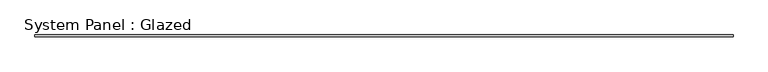
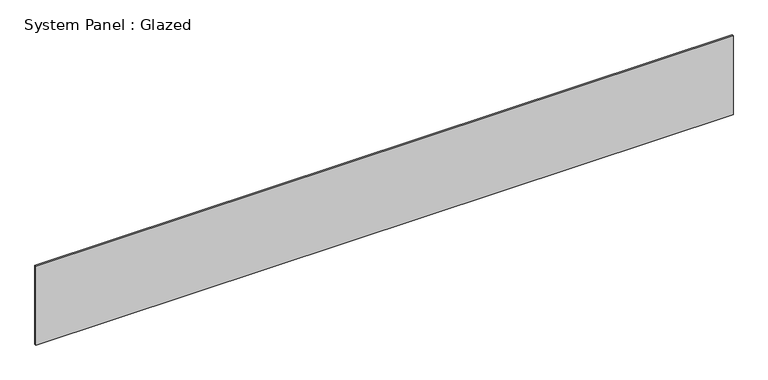
"""IFC4 building model written with IfcOpenShell, lengths in millimetres: plate geometry, System Panel : Glazed."""

from ifc_helpers import new_model, si_unit, origin, origin_with_axes, place, context, project, spatial, polyline, outline, extrude, source, transform, mapped, element, save


def system_panel_glazed_524a14c5(model_context):
    return source(origin(), model_context, "Body", "SweptSolid", [
        extrude(outline(polyline([(5105.4, 19.05), (-5105.4, 19.05), (-5105.4, 44.45), (5105.4, 44.45), (5105.4, 19.05)])), origin_with_axes(), (0.0, 0.0, 1.0), 1219.2),
    ])


if __name__ == "__main__":
    model = new_model("IFC4")
    model_context = context("Model", 3, world=origin())
    ifc_project = project(units=[si_unit("LENGTHUNIT", "METRE", prefix="MILLI")], contexts=[model_context])
    site = spatial("IfcSite", under=ifc_project)
    building = spatial("IfcBuilding", under=site)
    placement = place(None, origin())
    system_panel_glazed_shape = system_panel_glazed_524a14c5(model_context)
    element("IfcPlate", 1, ObjectType="System Panel : Glazed", at=placement, inside=building, context=model_context, shape_type="MappedRepresentation", body=[
        mapped(system_panel_glazed_shape, transform((0.0, 0.0, 0.0), x_axis=(1.0, 0.0, 0.0), y_axis=(0.0, 1.0, 0.0), z_axis=(0.0, 0.0, 1.0))),
    ])
    save(model, "model.ifc")

# Revit data of these elements
# Type "System Panel : Glazed"
#   Construction Type Id = "GSP4R"
#   Analytic Construction = "1/8 in Pilkington single glazing"
#   Visual Light Transmittance = 0.9
#   Solar Heat Gain Coefficient = 0.86
#   Heat Transfer Coefficient (U) = 1.18115 BTU/(h·ft²·°F)
# Element 1 (IfcPlate, "System Panel : Glazed")
#   Materials on its faces: "Glass"
# Materials
#   "Glass": class "Glass", colour RGB 0 128 192, transparency 0.75, Description = "Soda Lime Glass", Cost = 0
